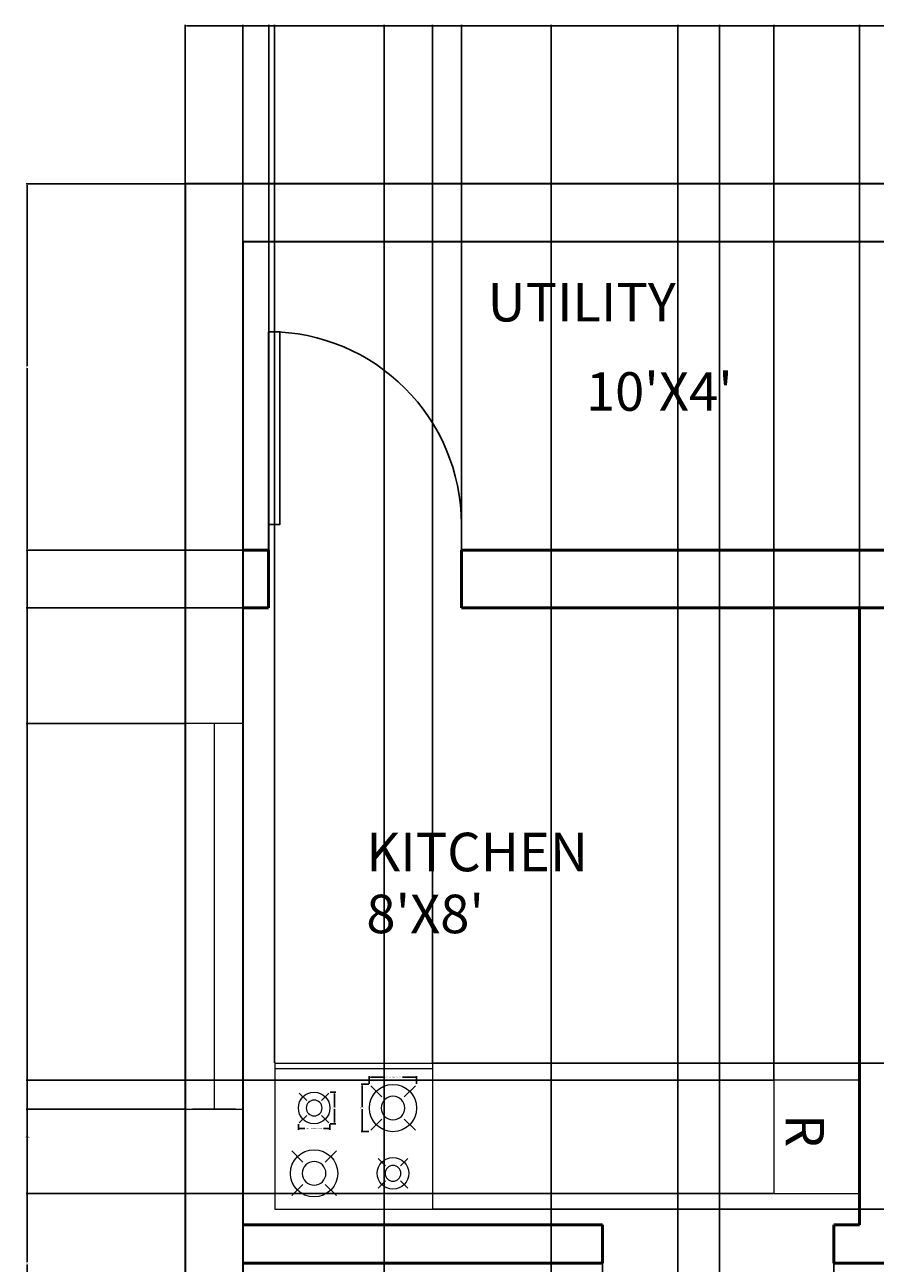
# Model space of a CAD drawing. Units: inches. Extents: x 8049 to 8459, y 820 to 1350.
# Tile 23 of 25: x 8049 to 8182, y 1157 to 1350. Entities that reach past the tile are written whole.
import ezdxf

# ---------------------------------------------------------------- set-up
doc = ezdxf.new("R2010")
doc.units = ezdxf.units.IN
doc.header["$MEASUREMENT"] = 0
for name, color, linetype, lineweight in [('A-ANNO-DIMS', 2, 'Continuous', 18), ('A-ANNO-TEXT', 7, 'Continuous', 18), ('A-AREA-IDEN', 7, 'Continuous', 25), ('A-DOOR', 3, 'Continuous', 25), ('A-EQPM', 8, 'Continuous', 18), ('A-GLAZ', 4, 'Continuous', 18), ('A-WALL', 7, 'Continuous', 50), ('C-SITE-WALL', 7, 'Continuous', 35)]:
    doc.layers.add(name, color=color, linetype=linetype, lineweight=lineweight)
doc.styles.get("Standard").update_dxf_attribs({"font": 'arial.ttf'})
doc.dimstyles.get("Standard").update_dxf_attribs({"dimtxt": 0.18, "dimasz": 0.18, "dimexe": 0.18, "dimexo": 0.0625, "dimgap": 0.09, "dimtad": 0, "dimtih": 1, "dimtoh": 1, "dimdec": 4, "dimzin": 0, "dimdsep": 46, "dimtxsty": 'Standard', "dimcen": 0.09, "dimadec": 0, "dimazin": 0, "dimtfac": 1, "dimtdec": 4, "dimtofl": 0, "dimtmove": 0, "dimatfit": 3, "dimfxl": 1, "dimtolj": 1, "dimtzin": 0, "dimarcsym": 0})

# ---------------------------------------------------------------- blocks, each defined once
blk = doc.blocks.new('*U2')
for p, q in [((0, 0), (0, -100)), ((750, 0), (750, -100))]:
    blk.add_line(p, q)
blk.add_lwpolyline([(0, 0), (0, 750), (43.75, 750), (43.75, 0)], close=True)
blk.add_arc((0, 0), 750, 0, 90)
blk = doc.blocks.new('*U4')
for p, q in [((0, 100), (0, 0)), ((900, 100), (900, 0)), ((0, 50), (900, 50))]:
    blk.add_line(p, q)
blk = doc.blocks.new('RANGE-BURNER-SMALL')
for p, q in [((1.3, 3.61), (0.14, 4.77)), ((3.61, 3.61), (4.77, 4.77)), ((1.3, 1.3), (0.14, 0.14)), ((3.61, 1.3), (4.77, 0.14))]:
    blk.add_line(p, q)
blk.add_circle((2.46, 2.46), 2.46)
for start, end in [(0, 180), (180, 0)]:
    blk.add_arc((2.46, 2.46), 1.23, start, end)
blk = doc.blocks.new('RANGE-BURNER-LARGE')
for p, q in [((1.95, 5.42), (0.21, 7.16)), ((5.42, 5.42), (7.16, 7.16)), ((1.95, 1.95), (0.21, 0.21)), ((5.42, 1.95), (7.16, 0.21))]:
    blk.add_line(p, q)
blk.add_circle((3.68, 3.68), 3.68)
for start, end in [(0, 180), (180, 0)]:
    blk.add_arc((3.68, 3.68), 1.84, start, end)
blk = doc.blocks.new('*D38')
at = {"layer": 'A-ANNO-DIMS', "color": 0, "lineweight": -2, "transparency": 16777216}
for p, q in [((8092.02, 1178.51), (8092.02, 1177.66)), ((8096.93, 1178.51), (8096.93, 1177.66)), ((8092.2, 1177.84), (8093.01, 1177.84)), ((8096.75, 1177.84), (8095.95, 1177.84))]:
    blk.add_line(p, q, dxfattribs=at)
at = {"layer": 'A-ANNO-DIMS', "color": 0, "transparency": 16777216}
for points in [[(8092.2, 1177.87), (8092.2, 1177.81), (8092.02, 1177.84)], [(8096.75, 1177.87), (8096.75, 1177.81), (8096.93, 1177.84)]]:
    blk.add_solid(points, dxfattribs=at)
at = {"layer": 'Defpoints', "color": 0, "transparency": 16777216}
for p in [(8092.02, 1178.58), (8096.93, 1178.58), (8096.93, 1177.84)]:
    blk.add_point(p, dxfattribs=at)
at = {"layer": 'A-ANNO-DIMS', "color": 0, "transparency": 16777216, "insert": (8094.48, 1177.84), "char_height": 0.18, "attachment_point": 5}
blk.add_mtext('\\A1;SMALL BURNER 5 TYP.', dxfattribs=at)
blk = doc.blocks.new('*D39')
at = {"layer": 'A-ANNO-DIMS', "color": 0, "lineweight": -2, "transparency": 16777216}
for p, q in [((8096.99, 1183.49), (8097.85, 1183.49)), ((8097.67, 1183.31), (8097.67, 1181.22)), ((8097.67, 1178.76), (8097.67, 1180.85)), ((8096.99, 1178.58), (8097.85, 1178.58))]:
    blk.add_line(p, q, dxfattribs=at)
at = {"layer": 'A-ANNO-DIMS', "color": 0, "transparency": 16777216}
for points in [[(8097.64, 1183.31), (8097.7, 1183.31), (8097.67, 1183.49)], [(8097.64, 1178.76), (8097.7, 1178.76), (8097.67, 1178.58)]]:
    blk.add_solid(points, dxfattribs=at)
at = {"layer": 'Defpoints', "color": 0, "transparency": 16777216}
for p in [(8096.93, 1183.49), (8097.67, 1183.49), (8096.93, 1178.58)]:
    blk.add_point(p, dxfattribs=at)
at = {"layer": 'A-ANNO-DIMS', "color": 0, "transparency": 16777216, "insert": (8097.67, 1181.03), "char_height": 0.18, "attachment_point": 5}
blk.add_mtext('\\A1;5 TYP.', dxfattribs=at)
blk = doc.blocks.new('*D40')
at = {"layer": 'A-ANNO-DIMS', "color": 0, "lineweight": -2, "transparency": 16777216}
for p, q in [((8103.07, 1184.78), (8103.07, 1186)), ((8103.25, 1185.82), (8105.28, 1185.82)), ((8110.26, 1185.82), (8108.24, 1185.82)), ((8110.44, 1184.78), (8110.44, 1186))]:
    blk.add_line(p, q, dxfattribs=at)
at = {"layer": 'A-ANNO-DIMS', "color": 0, "transparency": 16777216}
for points in [[(8103.25, 1185.85), (8103.25, 1185.79), (8103.07, 1185.82)], [(8110.26, 1185.85), (8110.26, 1185.79), (8110.44, 1185.82)]]:
    blk.add_solid(points, dxfattribs=at)
at = {"layer": 'Defpoints', "color": 0, "transparency": 16777216}
for p in [(8110.44, 1185.82), (8103.07, 1184.72), (8110.44, 1184.72)]:
    blk.add_point(p, dxfattribs=at)
at = {"layer": 'A-ANNO-DIMS', "color": 0, "transparency": 16777216, "insert": (8106.76, 1185.82), "char_height": 0.18, "attachment_point": 5}
blk.add_mtext('\\A1;LARGE BURNER 7 TYP.', dxfattribs=at)
blk = doc.blocks.new('*D41')
at = {"layer": 'A-ANNO-DIMS', "color": 0, "lineweight": -2, "transparency": 16777216}
for p, q in [((8103.01, 1184.72), (8101.79, 1184.72)), ((8101.97, 1184.54), (8101.97, 1181.21)), ((8101.97, 1177.53), (8101.97, 1180.85)), ((8103.01, 1177.35), (8101.79, 1177.35))]:
    blk.add_line(p, q, dxfattribs=at)
at = {"layer": 'A-ANNO-DIMS', "color": 0, "transparency": 16777216}
for points in [[(8101.94, 1184.54), (8102, 1184.54), (8101.97, 1184.72)], [(8101.94, 1177.53), (8102, 1177.53), (8101.97, 1177.35)]]:
    blk.add_solid(points, dxfattribs=at)
at = {"layer": 'Defpoints', "color": 0, "transparency": 16777216}
for p in [(8101.97, 1184.72), (8103.07, 1184.72), (8103.07, 1177.35)]:
    blk.add_point(p, dxfattribs=at)
at = {"layer": 'A-ANNO-DIMS', "color": 0, "transparency": 16777216, "insert": (8101.97, 1181.03), "char_height": 0.18, "attachment_point": 5}
blk.add_mtext('\\A1;7 TYP.', dxfattribs=at)
blk = doc.blocks.new('*D48')
at = {"layer": 'A-ANNO-DIMS', "color": 0, "lineweight": -2, "transparency": 16777216}
for p, q in [((8074.4, 1324.93), (8074.4, 1349.65)), ((8074.58, 1349.47), (8254.11, 1349.47)), ((8434.22, 1349.47), (8254.69, 1349.47)), ((8434.4, 1324.93), (8434.4, 1349.65))]:
    blk.add_line(p, q, dxfattribs=at)
at = {"layer": 'A-ANNO-DIMS', "color": 0, "transparency": 16777216}
for points in [[(8074.58, 1349.5), (8074.58, 1349.44), (8074.4, 1349.47)], [(8434.22, 1349.5), (8434.22, 1349.44), (8434.4, 1349.47)]]:
    blk.add_solid(points, dxfattribs=at)
at = {"layer": 'Defpoints', "color": 0, "transparency": 16777216}
for p in [(8434.4, 1349.47), (8074.4, 1324.87), (8434.4, 1324.87)]:
    blk.add_point(p, dxfattribs=at)
at = {"layer": 'A-ANNO-DIMS', "color": 0, "transparency": 16777216, "insert": (8254.4, 1349.47), "char_height": 0.18, "attachment_point": 5}
blk.add_mtext('\\A1;360', dxfattribs=at)
blk = doc.blocks.new('*D51')
at = {"layer": 'A-ANNO-DIMS', "color": 0, "lineweight": -2, "transparency": 16777216}
for p, q in [((8083.33, 1267.87), (8049.62, 1267.87)), ((8049.8, 1267.69), (8049.8, 1157.05)), ((8049.8, 1046.05), (8049.8, 1156.69)), ((8083.33, 1045.87), (8049.62, 1045.87))]:
    blk.add_line(p, q, dxfattribs=at)
at = {"layer": 'A-ANNO-DIMS', "color": 0, "transparency": 16777216}
for points in [[(8049.77, 1267.69), (8049.83, 1267.69), (8049.8, 1267.87)], [(8049.77, 1046.05), (8049.83, 1046.05), (8049.8, 1045.87)]]:
    blk.add_solid(points, dxfattribs=at)
at = {"layer": 'Defpoints', "color": 0, "transparency": 16777216}
for p in [(8049.8, 1267.87), (8083.4, 1267.87), (8083.4, 1045.87)]:
    blk.add_point(p, dxfattribs=at)
at = {"layer": 'A-ANNO-DIMS', "color": 0, "transparency": 16777216, "insert": (8049.8, 1156.87), "char_height": 0.18, "attachment_point": 5}
blk.add_mtext('\\A1;222', dxfattribs=at)
blk = doc.blocks.new('*D52')
at = {"layer": 'A-ANNO-DIMS', "color": 0, "lineweight": -2, "transparency": 16777216}
for p, q in [((8074.33, 1324.87), (8049.62, 1324.87)), ((8049.8, 1324.69), (8049.8, 1296.55)), ((8049.8, 1268.05), (8049.8, 1296.19)), ((8083.33, 1267.87), (8049.62, 1267.87))]:
    blk.add_line(p, q, dxfattribs=at)
at = {"layer": 'A-ANNO-DIMS', "color": 0, "transparency": 16777216}
for points in [[(8049.77, 1324.69), (8049.83, 1324.69), (8049.8, 1324.87)], [(8049.77, 1268.05), (8049.83, 1268.05), (8049.8, 1267.87)]]:
    blk.add_solid(points, dxfattribs=at)
at = {"layer": 'Defpoints', "color": 0, "transparency": 16777216}
for p in [(8049.8, 1324.87), (8074.4, 1324.87), (8083.4, 1267.87)]:
    blk.add_point(p, dxfattribs=at)
at = {"layer": 'A-ANNO-DIMS', "color": 0, "transparency": 16777216, "insert": (8049.8, 1296.37), "char_height": 0.18, "attachment_point": 5}
blk.add_mtext('\\A1;57', dxfattribs=at)
blk = doc.blocks.new('*D57')
at = {"layer": 'A-ANNO-DIMS', "color": 0, "lineweight": -2, "transparency": 16777216}
for p, q in [((8087.4, 1267.93), (8087.4, 1349.65)), ((8087.58, 1349.47), (8102.18, 1349.47)), ((8117.22, 1349.47), (8102.62, 1349.47)), ((8117.4, 1267.93), (8117.4, 1349.65))]:
    blk.add_line(p, q, dxfattribs=at)
at = {"layer": 'A-ANNO-DIMS', "color": 0, "transparency": 16777216}
for points in [[(8087.58, 1349.5), (8087.58, 1349.44), (8087.4, 1349.47)], [(8117.22, 1349.5), (8117.22, 1349.44), (8117.4, 1349.47)]]:
    blk.add_solid(points, dxfattribs=at)
at = {"layer": 'Defpoints', "color": 0, "transparency": 16777216}
for p in [(8117.4, 1349.47), (8087.4, 1267.87), (8117.4, 1267.87)]:
    blk.add_point(p, dxfattribs=at)
at = {"layer": 'A-ANNO-DIMS', "color": 0, "transparency": 16777216, "insert": (8102.4, 1349.47), "char_height": 0.18, "attachment_point": 5}
blk.add_mtext('\\A1;30', dxfattribs=at)
blk = doc.blocks.new('*D58')
at = {"layer": 'A-ANNO-DIMS', "color": 0, "lineweight": -2, "transparency": 16777216}
for p, q in [((8139.4, 1162.81), (8139.4, 820.09)), ((8175.4, 1162.81), (8175.4, 820.09)), ((8139.58, 820.27), (8157.18, 820.27)), ((8175.22, 820.27), (8157.62, 820.27))]:
    blk.add_line(p, q, dxfattribs=at)
at = {"layer": 'A-ANNO-DIMS', "color": 0, "transparency": 16777216}
for points in [[(8139.58, 820.3), (8139.58, 820.24), (8139.4, 820.27)], [(8175.22, 820.3), (8175.22, 820.24), (8175.4, 820.27)]]:
    blk.add_solid(points, dxfattribs=at)
at = {"layer": 'Defpoints', "color": 0, "transparency": 16777216}
for p in [(8139.4, 1162.87), (8175.4, 1162.87), (8175.4, 820.27)]:
    blk.add_point(p, dxfattribs=at)
at = {"layer": 'A-ANNO-DIMS', "color": 0, "transparency": 16777216, "insert": (8157.4, 820.27), "char_height": 0.18, "attachment_point": 5}
blk.add_mtext('\\A1;36', dxfattribs=at)
blk = doc.blocks.new('*D59')
at = {"layer": 'A-ANNO-DIMS', "color": 0, "lineweight": -2, "transparency": 16777216}
for p, q in [((8083.4, 925.93), (8083.4, 1349.65)), ((8083.58, 1349.47), (8107.17, 1349.47)), ((8131.22, 1349.47), (8107.62, 1349.47)), ((8131.4, 925.93), (8131.4, 1349.65))]:
    blk.add_line(p, q, dxfattribs=at)
at = {"layer": 'A-ANNO-DIMS', "color": 0, "transparency": 16777216}
for points in [[(8083.58, 1349.5), (8083.58, 1349.44), (8083.4, 1349.47)], [(8131.22, 1349.5), (8131.22, 1349.44), (8131.4, 1349.47)]]:
    blk.add_solid(points, dxfattribs=at)
at = {"layer": 'Defpoints', "color": 0, "transparency": 16777216}
for p in [(8131.4, 1349.47), (8083.4, 925.87), (8131.4, 925.87)]:
    blk.add_point(p, dxfattribs=at)
at = {"layer": 'A-ANNO-DIMS', "color": 0, "transparency": 16777216, "insert": (8107.4, 1349.47), "char_height": 0.18, "attachment_point": 5}
blk.add_mtext('\\A1;48', dxfattribs=at)
blk = doc.blocks.new('*D62')
at = {"layer": 'A-ANNO-DIMS', "color": 0, "lineweight": -2, "transparency": 16777216}
for p, q in [((8074.33, 1240.87), (8049.62, 1240.87)), ((8049.8, 1240.69), (8049.8, 1211.05)), ((8049.8, 1181.05), (8049.8, 1210.69)), ((8074.33, 1180.87), (8049.62, 1180.87))]:
    blk.add_line(p, q, dxfattribs=at)
at = {"layer": 'A-ANNO-DIMS', "color": 0, "transparency": 16777216}
for points in [[(8049.77, 1240.69), (8049.83, 1240.69), (8049.8, 1240.87)], [(8049.77, 1181.05), (8049.83, 1181.05), (8049.8, 1180.87)]]:
    blk.add_solid(points, dxfattribs=at)
at = {"layer": 'Defpoints', "color": 0, "transparency": 16777216}
for p in [(8049.8, 1240.87), (8074.4, 1240.87), (8074.4, 1180.87)]:
    blk.add_point(p, dxfattribs=at)
at = {"layer": 'A-ANNO-DIMS', "color": 0, "transparency": 16777216, "insert": (8049.8, 1210.87), "char_height": 0.18, "attachment_point": 5}
blk.add_mtext('\\A1;60', dxfattribs=at)
blk = doc.blocks.new('*D63')
at = {"layer": 'A-ANNO-DIMS', "color": 0, "lineweight": -2, "transparency": 16777216}
for p, q in [((8083.33, 1258.87), (8049.62, 1258.87)), ((8049.8, 1258.69), (8049.8, 1250.05)), ((8049.8, 1241.05), (8049.8, 1249.69)), ((8074.33, 1240.87), (8049.62, 1240.87))]:
    blk.add_line(p, q, dxfattribs=at)
at = {"layer": 'A-ANNO-DIMS', "color": 0, "transparency": 16777216}
for points in [[(8049.77, 1258.69), (8049.83, 1258.69), (8049.8, 1258.87)], [(8049.77, 1241.05), (8049.83, 1241.05), (8049.8, 1240.87)]]:
    blk.add_solid(points, dxfattribs=at)
at = {"layer": 'Defpoints', "color": 0, "transparency": 16777216}
for p in [(8049.8, 1258.87), (8083.4, 1258.87), (8074.4, 1240.87)]:
    blk.add_point(p, dxfattribs=at)
at = {"layer": 'A-ANNO-DIMS', "color": 0, "transparency": 16777216, "insert": (8049.8, 1249.87), "char_height": 0.18, "attachment_point": 5}
blk.add_mtext('\\A1;18', dxfattribs=at)
blk = doc.blocks.new('*D78')
at = {"layer": 'A-ANNO-DIMS', "color": 0, "lineweight": -2, "transparency": 16777216}
for p, q in [((8105.39, 1082.37), (8105.39, 1349.65)), ((8105.57, 1349.47), (8127.86, 1349.47)), ((8150.94, 1349.47), (8128.65, 1349.47)), ((8151.12, 1082.37), (8151.12, 1349.65))]:
    blk.add_line(p, q, dxfattribs=at)
at = {"layer": 'A-ANNO-DIMS', "color": 0, "transparency": 16777216}
for points in [[(8105.57, 1349.5), (8105.57, 1349.44), (8105.39, 1349.47)], [(8150.94, 1349.5), (8150.94, 1349.44), (8151.12, 1349.47)]]:
    blk.add_solid(points, dxfattribs=at)
at = {"layer": 'Defpoints', "color": 0, "transparency": 16777216}
for p in [(8151.12, 1349.47), (8105.39, 1082.31), (8151.12, 1082.31)]:
    blk.add_point(p, dxfattribs=at)
at = {"layer": 'A-ANNO-DIMS', "color": 0, "transparency": 16777216, "insert": (8128.25, 1349.47), "char_height": 0.18, "attachment_point": 5}
blk.add_mtext('\\A1;45.72', dxfattribs=at)
blk = doc.blocks.new('*D79')
at = {"layer": 'A-ANNO-DIMS', "color": 0, "lineweight": -2, "transparency": 16777216}
for p, q in [((8157.59, 1082.57), (8157.59, 1349.65)), ((8157.77, 1349.47), (8183.11, 1349.47)), ((8209.23, 1349.47), (8183.9, 1349.47)), ((8209.41, 1082.57), (8209.41, 1349.65))]:
    blk.add_line(p, q, dxfattribs=at)
at = {"layer": 'A-ANNO-DIMS', "color": 0, "transparency": 16777216}
for points in [[(8157.77, 1349.5), (8157.77, 1349.44), (8157.59, 1349.47)], [(8209.23, 1349.5), (8209.23, 1349.44), (8209.41, 1349.47)]]:
    blk.add_solid(points, dxfattribs=at)
at = {"layer": 'Defpoints', "color": 0, "transparency": 16777216}
for p in [(8209.41, 1349.47), (8157.59, 1082.51), (8209.41, 1082.51)]:
    blk.add_point(p, dxfattribs=at)
at = {"layer": 'A-ANNO-DIMS', "color": 0, "transparency": 16777216, "insert": (8183.5, 1349.47), "char_height": 0.18, "attachment_point": 5}
blk.add_mtext('\\A1;51.82', dxfattribs=at)
blk = doc.blocks.new('*D82')
at = {"layer": 'A-ANNO-DIMS', "color": 0, "lineweight": -2, "transparency": 16777216}
for p, q in [((8088.33, 1188.06), (8088.33, 1349.65)), ((8088.51, 1349.47), (8100.15, 1349.47)), ((8112.72, 1349.47), (8101.08, 1349.47)), ((8112.9, 1188.06), (8112.9, 1349.65))]:
    blk.add_line(p, q, dxfattribs=at)
at = {"layer": 'A-ANNO-DIMS', "color": 0, "transparency": 16777216}
for points in [[(8088.51, 1349.5), (8088.51, 1349.44), (8088.33, 1349.47)], [(8112.72, 1349.5), (8112.72, 1349.44), (8112.9, 1349.47)]]:
    blk.add_solid(points, dxfattribs=at)
at = {"layer": 'Defpoints', "color": 0, "transparency": 16777216}
for p in [(8112.9, 1349.47), (8088.33, 1187.99), (8112.9, 1187.99)]:
    blk.add_point(p, dxfattribs=at)
at = {"layer": 'A-ANNO-DIMS', "color": 0, "transparency": 16777216, "insert": (8100.62, 1349.47), "char_height": 0.18, "attachment_point": 5}
blk.add_mtext('\\A1;24.566', dxfattribs=at)
blk = doc.blocks.new('*D83')
at = {"layer": 'A-ANNO-DIMS', "color": 0, "lineweight": -2, "transparency": 16777216}
for p, q in [((8112.96, 1187.99), (8459.18, 1187.99)), ((8459, 1187.81), (8459, 1176.83)), ((8459, 1165.49), (8459, 1176.47)), ((8112.96, 1165.31), (8459.18, 1165.31))]:
    blk.add_line(p, q, dxfattribs=at)
at = {"layer": 'A-ANNO-DIMS', "color": 0, "transparency": 16777216}
for points in [[(8458.97, 1187.81), (8459.03, 1187.81), (8459, 1187.99)], [(8458.97, 1165.49), (8459.03, 1165.49), (8459, 1165.31)]]:
    blk.add_solid(points, dxfattribs=at)
at = {"layer": 'Defpoints', "color": 0, "transparency": 16777216}
for p in [(8112.9, 1187.99), (8459, 1187.99), (8112.9, 1165.31)]:
    blk.add_point(p, dxfattribs=at)
at = {"layer": 'A-ANNO-DIMS', "color": 0, "transparency": 16777216, "insert": (8459, 1176.65), "char_height": 0.18, "attachment_point": 5}
blk.add_mtext('\\A1;22.68', dxfattribs=at)
blk = doc.blocks.new('*D84')
at = {"layer": 'A-ANNO-DIMS', "color": 0, "lineweight": -2, "transparency": 16777216}
for p, q in [((8166.03, 1185.42), (8166.03, 1349.65)), ((8166.21, 1349.47), (8172.26, 1349.47)), ((8179.22, 1349.47), (8173.17, 1349.47)), ((8179.4, 1185.42), (8179.4, 1349.65))]:
    blk.add_line(p, q, dxfattribs=at)
at = {"layer": 'A-ANNO-DIMS', "color": 0, "transparency": 16777216}
for points in [[(8166.21, 1349.5), (8166.21, 1349.44), (8166.03, 1349.47)], [(8179.22, 1349.5), (8179.22, 1349.44), (8179.4, 1349.47)]]:
    blk.add_solid(points, dxfattribs=at)
at = {"layer": 'Defpoints', "color": 0, "transparency": 16777216}
for p in [(8179.4, 1349.47), (8166.03, 1185.36), (8179.4, 1185.36)]:
    blk.add_point(p, dxfattribs=at)
at = {"layer": 'A-ANNO-DIMS', "color": 0, "transparency": 16777216, "insert": (8172.71, 1349.47), "char_height": 0.18, "attachment_point": 5}
blk.add_mtext('\\A1;13.372', dxfattribs=at)
blk = doc.blocks.new('*D85')
at = {"layer": 'A-ANNO-DIMS', "color": 0, "lineweight": -2, "transparency": 16777216}
for p, q in [((8165.96, 1185.36), (8049.62, 1185.36)), ((8049.8, 1185.18), (8049.8, 1176.71)), ((8049.8, 1167.89), (8049.8, 1176.35)), ((8165.96, 1167.71), (8049.62, 1167.71))]:
    blk.add_line(p, q, dxfattribs=at)
at = {"layer": 'A-ANNO-DIMS', "color": 0, "transparency": 16777216}
for points in [[(8049.77, 1185.18), (8049.83, 1185.18), (8049.8, 1185.36)], [(8049.77, 1167.89), (8049.83, 1167.89), (8049.8, 1167.71)]]:
    blk.add_solid(points, dxfattribs=at)
at = {"layer": 'Defpoints', "color": 0, "transparency": 16777216}
for p in [(8049.8, 1185.36), (8166.03, 1185.36), (8166.03, 1167.71)]:
    blk.add_point(p, dxfattribs=at)
at = {"layer": 'A-ANNO-DIMS', "color": 0, "transparency": 16777216, "insert": (8049.8, 1176.53), "char_height": 0.18, "attachment_point": 5}
blk.add_mtext('\\A1;17.652', dxfattribs=at)
blk = doc.blocks.new('*D88')
at = {"layer": 'A-ANNO-DIMS', "color": 0, "lineweight": -2, "transparency": 16777216}
for p, q in [((8083.4, 1162.81), (8083.4, 820.09)), ((8139.4, 1162.81), (8139.4, 820.09)), ((8083.58, 820.27), (8111.18, 820.27)), ((8139.22, 820.27), (8111.62, 820.27))]:
    blk.add_line(p, q, dxfattribs=at)
at = {"layer": 'A-ANNO-DIMS', "color": 0, "transparency": 16777216}
for points in [[(8083.58, 820.3), (8083.58, 820.24), (8083.4, 820.27)], [(8139.22, 820.3), (8139.22, 820.24), (8139.4, 820.27)]]:
    blk.add_solid(points, dxfattribs=at)
at = {"layer": 'Defpoints', "color": 0, "transparency": 16777216}
for p in [(8083.4, 1162.87), (8139.4, 1162.87), (8139.4, 820.27)]:
    blk.add_point(p, dxfattribs=at)
at = {"layer": 'A-ANNO-DIMS', "color": 0, "transparency": 16777216, "insert": (8111.4, 820.27), "char_height": 0.18, "attachment_point": 5}
blk.add_mtext('\\A1;56', dxfattribs=at)

msp = doc.modelspace()

# ---------------------------------------------------------------- linework, layer by layer
at = {"layer": 'A-EQPM'}
for p, q in [((8088.3346, 1187.9939), (8112.9001, 1187.9939)), ((8088.3346, 1187.9939), (8088.3346, 1165.3117)), ((8112.9001, 1187.9939), (8112.9001, 1165.3117)), ((8088.3346, 1187.175), (8112.9001, 1187.175)), ((8088.3346, 1165.3117), (8112.9001, 1165.3117))]:
    msp.add_line(p, q, dxfattribs=at)
msp.add_lwpolyline([(8179.3974, 1185.3584), (8166.0253, 1185.3584), (8166.0253, 1167.706), (8179.3974, 1167.706)], close=True, dxfattribs=at)
at = {"layer": 'A-GLAZ'}
for p, q in [((8083.3974, 1240.8706), (8074.3974, 1240.8706)), ((8074.3974, 1240.8706), (8074.3974, 1180.8706)), ((8074.3974, 1180.8706), (8083.3974, 1180.8706))]:
    msp.add_line(p, q, dxfattribs=at)
at = {"layer": 'A-WALL'}
for p, q in [((8087.3974, 1267.8706), (8083.3974, 1267.8706)), ((8087.3974, 1258.8706), (8087.3974, 1267.8706)), ((8425.3974, 1267.8706), (8117.3974, 1267.8706)), ((8117.3974, 1267.8706), (8117.3974, 1258.8706)), ((8083.3974, 1258.8706), (8087.3974, 1258.8706)), ((8117.3974, 1258.8706), (8425.3974, 1258.8706)), ((8179.3974, 1258.8706), (8179.3974, 1162.8706)), ((8083.3974, 1162.8706), (8139.3974, 1162.8706)), ((8139.3974, 1156.8706), (8139.3974, 1162.8706)), ((8175.3974, 1162.8706), (8175.3974, 1156.8706)), ((8175.3974, 1162.8706), (8179.3974, 1162.8706)), ((8083.3974, 1156.8706), (8139.3974, 1156.8706)), ((8175.3974, 1156.8706), (8205.3974, 1156.8706))]:
    msp.add_line(p, q, dxfattribs=at)
at = {"layer": 'C-SITE-WALL'}
for p, q in [((8434.3974, 1324.8706), (8074.3974, 1324.8706)), ((8074.3974, 1324.8706), (8074.3974, 844.8706)), ((8083.3974, 1315.8706), (8083.3974, 853.8706)), ((8425.3974, 1315.8706), (8083.3974, 1315.8706))]:
    msp.add_line(p, q, dxfattribs=at)

# ---------------------------------------------------------------- block references
at = {"layer": 'A-DOOR', "xscale": 0.0399999999999999, "yscale": 0.0399999999999999, "zscale": 0.0399999999999999}
msp.add_blockref('*U2', (8087.3974, 1271.8706), dxfattribs=at)
at = {"layer": 'A-EQPM'}
for name, p in [('RANGE-BURNER-LARGE', (8103.0738, 1177.3489)), ('RANGE-BURNER-SMALL', (8092.019, 1178.577)), ('RANGE-BURNER-LARGE', (8090.791, 1167.183))]:
    msp.add_blockref(name, p, dxfattribs=at)
at = {"layer": 'A-EQPM', "rotation": 180}
msp.add_blockref('RANGE-BURNER-SMALL', (8109.2157, 1173.3243), dxfattribs=at)
at = {"layer": 'A-GLAZ', "xscale": 0.0666666666666668, "yscale": 0.0666666666666668, "zscale": 0.0666666666666668, "rotation": 270}
msp.add_blockref('*U4', (8075.5641, 1240.8706), dxfattribs=at)

# ---------------------------------------------------------------- texts
at = {"layer": 'A-ANNO-TEXT'}
msp.add_text('R', height=6, rotation=270, dxfattribs=at).set_placement((8167.8779, 1180.099))
at = {"layer": 'A-AREA-IDEN'}
for s, p in [('UTILITY', (8121.4905, 1303.4647)), ("10'X4'", (8136.7902, 1289.5641)), ('KITCHEN', (8102.6025, 1217.8795)), ("8'X8'", (8102.6025, 1208.241))]:
    msp.add_text(s, height=6, dxfattribs=at).set_placement(p)

# ---------------------------------------------------------------- dimensions: what is measured, and where the dimension line sits
at = {"layer": 'A-ANNO-DIMS'}
for base, p1, p2, override, picture, middle in [((8434.3974, 1349.4706), (8074.3974, 1324.8706), (8434.3974, 1324.8706), {"dimdec": 0, "dimlfac": 1, "dimrnd": 0, "dimzin": 0, "dimdsep": 46, "dimlunit": 2}, '*D48', (8254.3974, 1349.4706)), ((8131.3974, 1349.4706), (8083.3974, 925.8706), (8131.3974, 925.8706), {"dimdec": 0, "dimlfac": 1, "dimrnd": 0, "dimzin": 0, "dimdsep": 46, "dimlunit": 2}, '*D59', (8107.3974, 1349.4706)), ((8117.3974, 1349.4706), (8087.3974, 1267.8706), (8117.3974, 1267.8706), {"dimdec": 0, "dimlfac": 1, "dimrnd": 0, "dimzin": 0, "dimdsep": 46, "dimlunit": 2}, '*D57', (8102.3974, 1349.4706)), ((8112.9001, 1349.47061), (8088.33455, 1187.99387), (8112.9001, 1187.99387), {"dimdec": 3, "dimlfac": 1, "dimrnd": 0, "dimzin": 0, "dimdsep": 46, "dimlunit": 2}, '*D82', (8100.61732, 1349.47061)), ((8151.1153, 1349.4706), (8105.3911, 1082.3072), (8151.1153, 1082.3072), {"dimdec": 2, "dimlfac": 1, "dimrnd": 0, "dimzin": 0, "dimdsep": 46, "dimlunit": 2}, '*D78', (8128.2532, 1349.4706)), ((8209.4146, 1349.4706), (8157.5937, 1082.5119), (8209.4146, 1082.5119), {"dimdec": 2, "dimlfac": 1, "dimrnd": 0, "dimzin": 0, "dimdsep": 46, "dimlunit": 2}, '*D79', (8183.5041, 1349.4706)), ((8179.3974, 1349.4706), (8166.0253, 1185.3584), (8179.3974, 1185.3584), {"dimdec": 3, "dimlfac": 1, "dimrnd": 0, "dimzin": 0, "dimdsep": 46, "dimlunit": 2}, '*D84', (8172.7114, 1349.4706)), ((8139.3974, 820.2706), (8083.3974, 1162.8706), (8139.3974, 1162.8706), {"dimdec": 0, "dimlfac": 1, "dimrnd": 0, "dimzin": 0, "dimdsep": 46, "dimlunit": 2}, '*D88', (8111.3974, 820.2706)), ((8175.3974, 820.2706), (8139.3974, 1162.8706), (8175.3974, 1162.8706), {"dimdec": 0, "dimlfac": 1, "dimrnd": 0, "dimzin": 0, "dimdsep": 46, "dimlunit": 2}, '*D58', (8157.3974, 820.2706))]:
    dim = msp.add_linear_dim(base=base, p1=p1, p2=p2, dimstyle='Standard', override=override, dxfattribs=at)
    dim.commit()
    dim.dimension.update_dxf_attribs({"geometry": picture, "text_midpoint": middle})
for base, p1, p2, override, picture, middle in [((8049.7974, 1324.8706), (8083.3974, 1267.8706), (8074.3974, 1324.8706), {"dimdec": 0, "dimlfac": 1, "dimrnd": 0, "dimzin": 0, "dimdsep": 46, "dimlunit": 2}, '*D52', (8049.7974, 1296.3706)), ((8049.7974, 1267.8706), (8083.3974, 1045.8706), (8083.3974, 1267.8706), {"dimdec": 0, "dimlfac": 1, "dimrnd": 0, "dimzin": 0, "dimdsep": 46, "dimlunit": 2}, '*D51', (8049.7974, 1156.8706)), ((8049.7974, 1258.8706), (8074.3974, 1240.8706), (8083.3974, 1258.8706), {"dimdec": 0, "dimlfac": 1, "dimrnd": 0, "dimzin": 0, "dimdsep": 46, "dimlunit": 2}, '*D63', (8049.7974, 1249.8706)), ((8049.7974, 1240.8706), (8074.3974, 1180.8706), (8074.3974, 1240.8706), {"dimdec": 0, "dimlfac": 1, "dimrnd": 0, "dimzin": 0, "dimdsep": 46, "dimlunit": 2}, '*D62', (8049.7974, 1210.8706)), ((8458.9974, 1187.9939), (8112.9001, 1165.3117), (8112.9001, 1187.9939), {"dimdec": 2, "dimlfac": 1, "dimrnd": 0, "dimzin": 0, "dimdsep": 46, "dimlunit": 2}, '*D83', (8458.9974, 1176.6528)), ((8049.7974, 1185.3584), (8166.0253, 1167.706), (8166.0253, 1185.3584), {"dimdec": 3, "dimlfac": 1, "dimrnd": 0, "dimzin": 0, "dimdsep": 46, "dimlunit": 2}, '*D85', (8049.7974, 1176.5322))]:
    dim = msp.add_linear_dim(base=base, p1=p1, p2=p2, angle=90, dimstyle='Standard', override=override, dxfattribs=at)
    dim.commit()
    dim.dimension.update_dxf_attribs({"geometry": picture, "text_midpoint": middle})
for base, p1, p2, text, picture, middle in [((8110.4435, 1185.8239), (8103.0739, 1184.7185), (8110.4435, 1184.7185), 'LARGE BURNER <> TYP.', '*D40', (8106.7587, 1185.8239)), ((8096.9325, 1177.8401), (8092.0194, 1178.5771), (8096.9325, 1178.5771), 'SMALL BURNER <> TYP.', '*D38', (8094.4759, 1177.8401))]:
    dim = msp.add_linear_dim(base=base, p1=p1, p2=p2, text=text, dimstyle='Standard', override={"dimdec": 0, "dimlfac": 1, "dimrnd": 0, "dimzin": 0, "dimdsep": 46, "dimlunit": 2}, dxfattribs=at)
    dim.commit()
    dim.dimension.update_dxf_attribs({"geometry": picture, "text_midpoint": middle})
for base, p1, p2, picture, middle in [((8101.9684, 1184.7185), (8103.0739, 1177.3488), (8103.0739, 1184.7185), '*D41', (8101.9684, 1181.0336)), ((8097.6695, 1183.4902), (8096.9325, 1178.5771), (8096.9325, 1183.4902), '*D39', (8097.6695, 1181.0336))]:
    dim = msp.add_linear_dim(base=base, p1=p1, p2=p2, angle=90, text='<> TYP.', dimstyle='Standard', override={"dimdec": 0, "dimlfac": 1, "dimrnd": 0, "dimzin": 0, "dimdsep": 46, "dimlunit": 2}, dxfattribs=at)
    dim.commit()
    dim.dimension.update_dxf_attribs({"geometry": picture, "text_midpoint": middle})

doc.saveas('drawing.dxf')
